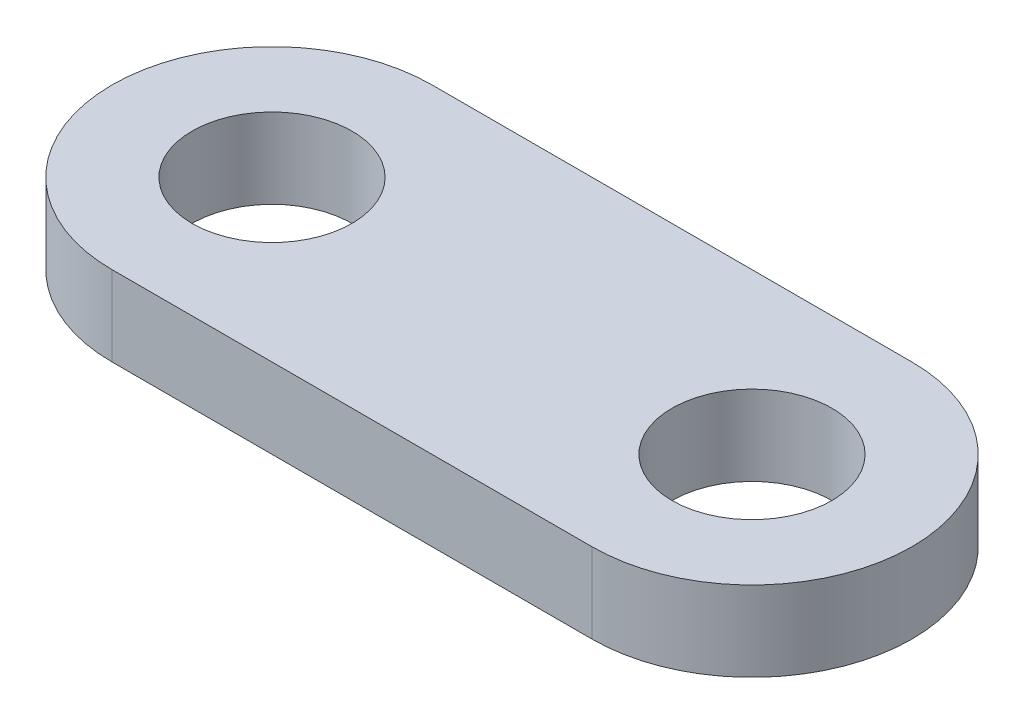
SolidWorks part; units mm, degrees
material "Plain Carbon Steel"
ref_plane "Front Plane" through (0, 0, 0) normal (0, 0, 1) x (1, 0, 0)
ref_plane "Top Plane" through (0, 0, 0) normal (0, 1, 0) x (1, 0, 0)
ref_plane "Right Plane" through (0, 0, 0) normal (1, 0, 0) x (0, 0, -1)
sketch "Link Profile" plane through (0, 0, 0) normal (0, 1, 0) x (1, 0, 0)
  line L0 (-15, 0) -> (15, 0) construction
  line L1 (-15, 10) -> (15, 10)
  line L2 (-15, -10) -> (15, -10)
  arc A0 (-15, 10) -> (-15, -10) centre (-15, 0) ccw
  arc A1 (15, -10) -> (15, 10) centre (15, 0) ccw
  circle A2 centre (-15, 0) radius 5
  circle A3 centre (15, 0) radius 5
  point P2 (0, 0)
  dimension "D2" = 10
  dimension "D3" = 10
  dimension "D1" = 30
extrude "Link Plate 5mm" add sketch "Link Profile" along normal blind 5
